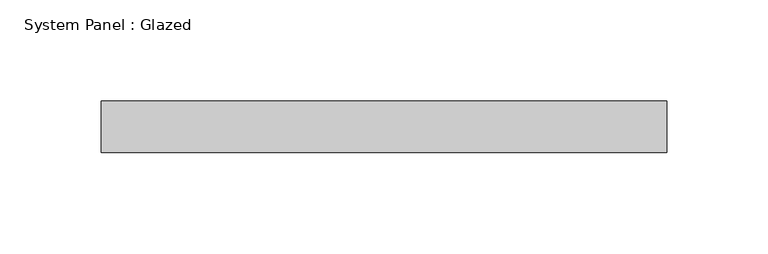
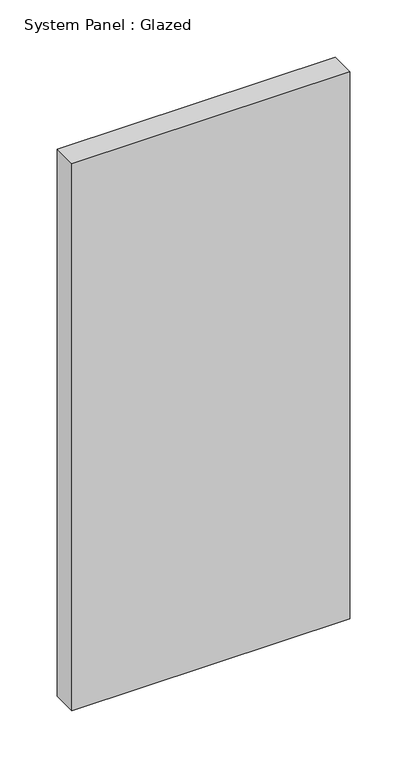
"""IFC4 building model written with IfcOpenShell, lengths in millimetres: plate geometry, System Panel : Glazed."""

from ifc_helpers import new_model, si_unit, origin, origin_with_axes, place, context, project, spatial, polyline, outline, extrude, source, transform, mapped, element, save


def system_panel_glazed_2307425d(model_context):
    return source(origin(), model_context, "Body", "SweptSolid", [
        extrude(outline(polyline([(139.7, 19.05), (-139.7, 19.05), (-139.7, 44.45), (139.7, 44.45), (139.7, 19.05)])), origin_with_axes(), (0.0, 0.0, 1.0), 581.769824),
    ])


if __name__ == "__main__":
    model = new_model("IFC4")
    model_context = context("Model", 3, world=origin())
    ifc_project = project(units=[si_unit("LENGTHUNIT", "METRE", prefix="MILLI")], contexts=[model_context])
    site = spatial("IfcSite", under=ifc_project)
    building = spatial("IfcBuilding", under=site)
    placement = place(None, origin())
    system_panel_glazed_shape = system_panel_glazed_2307425d(model_context)
    element("IfcPlate", 1, ObjectType="System Panel : Glazed", at=placement, inside=building, context=model_context, shape_type="MappedRepresentation", body=[
        mapped(system_panel_glazed_shape, transform((0.0, 0.0, 0.0), x_axis=(1.0, 0.0, 0.0), y_axis=(0.0, 1.0, 0.0), z_axis=(0.0, 0.0, 1.0))),
    ])
    save(model, "model.ifc")

# Revit data of these elements
# Type "System Panel : Glazed"
#   Construction Type Id = "GSP4R"
#   Analytic Construction = "1/8 in Pilkington single glazing"
#   Visual Light Transmittance = 0.9
#   Solar Heat Gain Coefficient = 0.86
#   Heat Transfer Coefficient (U) = 1.18115 BTU/(h·ft²·°F)
#   Define Thermal Properties by = 1
# Element 1 (IfcPlate, "System Panel : Glazed")
#   Materials on its faces: "Glass"
# Materials
#   "Glass": class "Glass", colour RGB 0 128 192, transparency 0.75, Description = "Soda Lime Glass", Cost = 0
